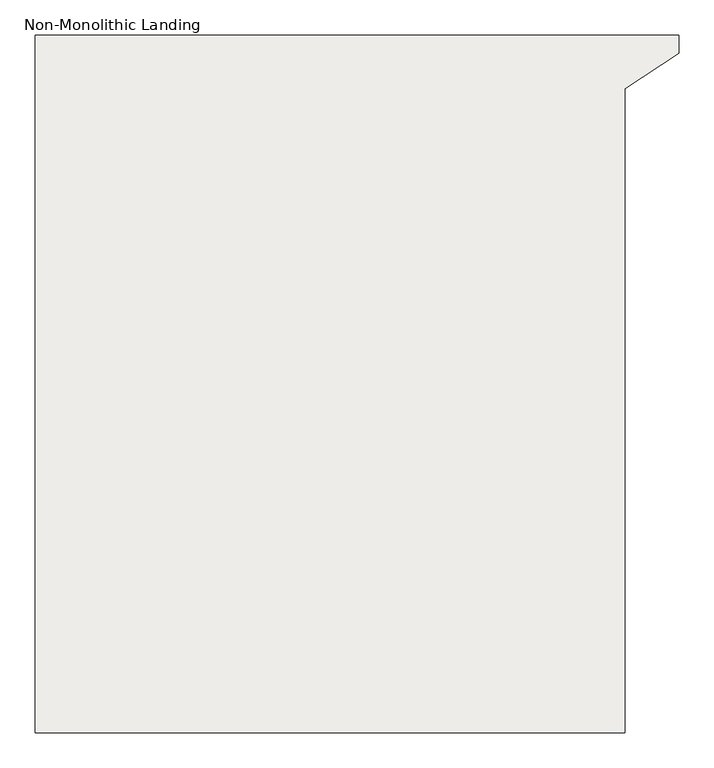
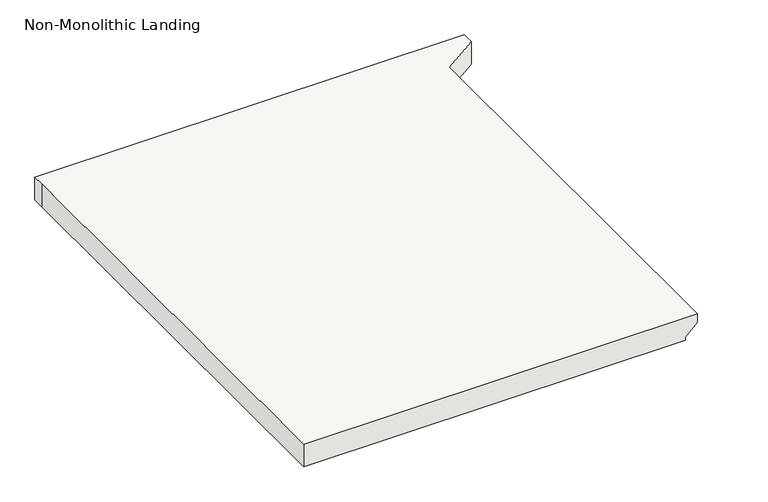
"""IFC4 building model written with IfcOpenShell, lengths in millimetres: slab geometry, Non-Monolithic Landing."""

from ifc_helpers import new_model, si_unit, origin, place, context, project, spatial, faceted_brep, source, transform, mapped, element, save


def non_monolithic_landing_8bb0a33a(model_context):
    return source(origin(), model_context, "Body", "Brep", [
        faceted_brep([(4353.0597674, -2307.0241735, 1016.0), (4353.0597674, -2307.0241735, 996.95), (4353.0597674, -1392.6241735, 996.95), (4353.0597674, -1392.6241735, 1016.0), (4327.6597674, -2307.0241735, 971.55), (4327.6597674, -1409.5575068, 971.55), (4429.2597674, -1341.8241735, 1016.0), (4429.2597674, -1316.4241735, 1016.0), (3514.8597674, -1316.4241735, 1016.0), (3514.8597674, -1341.8241735, 1016.0), (3514.8597674, -2307.0241735, 1016.0), (4327.6597674, -1409.5575068, 965.2), (4327.6597674, -2307.0241735, 965.2), (3514.8597674, -2307.0241735, 965.2), (3514.8597674, -1341.8241735, 965.2), (3514.8597674, -1316.4241735, 965.2), (4429.2597674, -1316.4241735, 965.2), (4429.2597674, -1341.8241735, 965.2)], [[[0, 1, 2, 3]], [[1, 4, 5, 2]], [[6, 7, 8, 9, 10, 0, 3]], [[11, 12, 13, 14, 15, 16, 17]], [[12, 11, 5, 4]], [[11, 17, 6, 3, 2, 5]], [[7, 6, 17, 16]], [[8, 7, 16, 15]], [[9, 8, 15, 14]], [[10, 9, 14, 13]], [[0, 10, 13, 12, 4, 1]]]),
    ])


if __name__ == "__main__":
    model = new_model("IFC4")
    model_context = context("Model", 3, world=origin())
    ifc_project = project(units=[si_unit("LENGTHUNIT", "METRE", prefix="MILLI")], contexts=[model_context])
    site = spatial("IfcSite", under=ifc_project)
    building = spatial("IfcBuilding", under=site)
    placement = place(None, origin())
    non_monolithic_landing_shape = non_monolithic_landing_8bb0a33a(model_context)
    element("IfcSlab", 1, ObjectType="Non-Monolithic Landing", at=placement, inside=building, context=model_context, shape_type="MappedRepresentation", body=[
        mapped(non_monolithic_landing_shape, transform((0.0, 0.0, 0.0), x_axis=(1.0, 0.0, 0.0), y_axis=(0.0, 1.0, 0.0), z_axis=(0.0, 0.0, 1.0))),
    ])
    save(model, "model.ifc")
